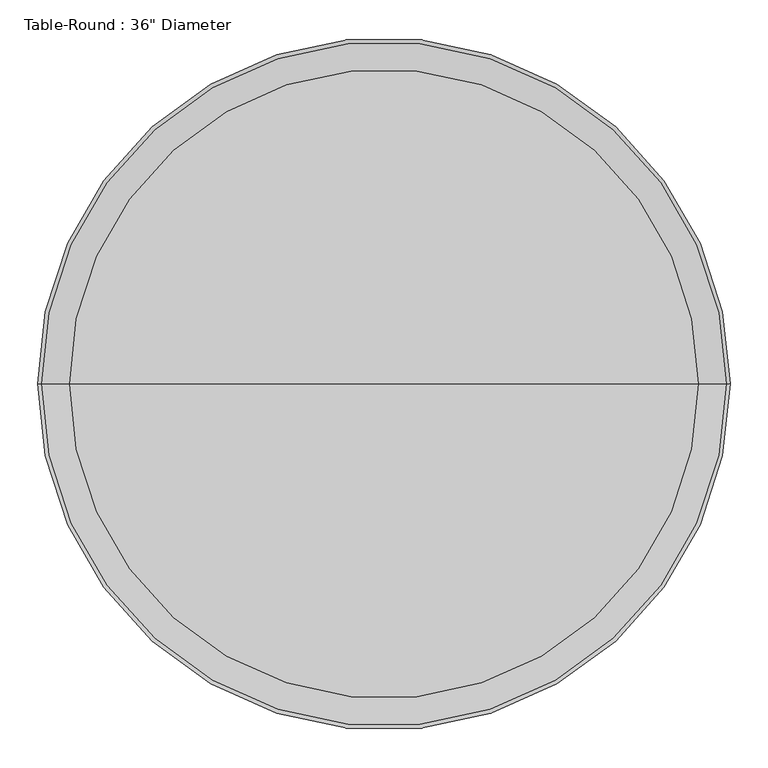
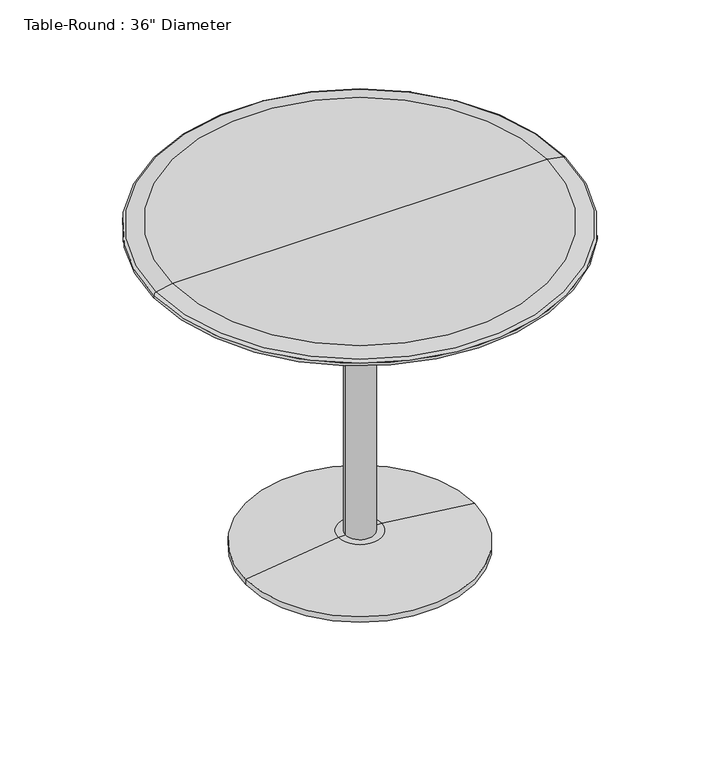
"""IFC4 building model written with IfcOpenShell, lengths in millimetres: furniture geometry."""

from ifc_helpers import new_model, si_unit, point, frame, origin, origin_2d, place, context, project, spatial, polyline, circle_curve, ellipse_curve, trimmed, segment, composite_curve, outline, extrude, source, transform, mapped, element, save
from ifc_brep_helpers import plane_surface, cylinder_surface, revolved_surface, advanced_brep


def furniture_c80d6d9c(model_context):
    return source(origin(), model_context, "Body", "SolidModel", [
        extrude(outline(composite_curve([segment(trimmed(circle_curve(origin_2d(), 31.75), [point((-31.75, 0.0))], [point((31.75, 0.0))], False, "CARTESIAN"), True, "CONTINUOUS"), segment(trimmed(circle_curve(origin_2d(), 31.75), [point((31.75, 0.0))], [point((-31.75, 0.0))], False, "CARTESIAN"), True, "CONTINUOUS")], self_intersect=False)), frame((0.0, 0.0, 38.1), z_axis=(0.0, 0.0, 1.0), x_axis=(1.0, 0.0, 0.0)), (0.0, 0.0, 1.0), 704.85),
        advanced_brep(
        [(0.0, 0.0, 742.95), (-457.2, 0.0, 742.95), (457.2, 0.0, 742.95), (415.3011364, 0.0, 762.0), (-415.3011364, 0.0, 762.0), (0.0, 0.0, 762.0), (451.9526659, 0.0, 755.5373465), (-451.9526659, 0.0, 755.5373465), (457.2, 0.0, 749.2838172), (-457.2, 0.0, 749.2838172)],
        [
            (0, 1),
            (1, 2, circle_curve(frame((0.0, 0.0, 742.95), z_axis=(0.0, 0.0, -1.0), x_axis=(-1.0, 0.0, 0.0)), 457.2)),
            (2, 0),
            (2, 1, circle_curve(frame((0.0, 0.0, 742.95), z_axis=(0.0, 0.0, -1.0), x_axis=(-1.0, 0.0, 0.0)), 457.2)),
            (3, 4, circle_curve(frame((0.0, 0.0, 762.0), z_axis=(0.0, 0.0, 1.0), x_axis=(-1.0, 0.0, 0.0)), 415.3011364)),
            (4, 5),
            (5, 3),
            (4, 3, circle_curve(frame((0.0, 0.0, 762.0), z_axis=(0.0, 0.0, 1.0), x_axis=(-1.0, 0.0, 0.0)), 415.3011364)),
            (6, 7, circle_curve(frame((0.0, 0.0, 755.5373465), z_axis=(0.0, 0.0, 1.0), x_axis=(-1.0, 0.0, 0.0)), 451.9526659)),
            (7, 4),
            (3, 6),
            (7, 6, circle_curve(frame((0.0, 0.0, 755.5373465), z_axis=(0.0, 0.0, 1.0), x_axis=(-1.0, 0.0, 0.0)), 451.9526659)),
            (8, 9, circle_curve(frame((0.0, 0.0, 749.2838172), z_axis=(0.0, 0.0, 1.0), x_axis=(-1.0, 0.0, 0.0)), 457.2)),
            (9, 7, circle_curve(frame((-450.85, 0.0, 749.2838172), z_axis=(0.0, 1.0, 0.0), x_axis=(1.0, 0.0, 0.0)), 6.35)),
            (6, 8, circle_curve(frame((450.85, 0.0, 749.2838172), z_axis=(0.0, 1.0, 0.0), x_axis=(-1.0, 0.0, 0.0)), 6.35)),
            (9, 8, circle_curve(frame((0.0, 0.0, 749.2838172), z_axis=(0.0, 0.0, 1.0), x_axis=(-1.0, 0.0, 0.0)), 457.2)),
            (1, 9),
            (8, 2),
        ],
        [
            plane_surface(frame((0.0, 0.0, 742.95), z_axis=(0.0, 0.0, -1.0), x_axis=(-1.0, 0.0, 0.0))),
            plane_surface(frame((0.0, 0.0, 762.0), z_axis=(0.0, 0.0, 1.0), x_axis=(-1.0, 0.0, 0.0))),
            revolved_surface(polyline([(-415.3011364, 0.0, 762.0), (-451.9526659, 0.0, 755.5373465)]), (0.0, 0.0, 838.2), (0.0, 0.0, -1.0)),
            revolved_surface(trimmed(ellipse_curve(frame((-450.85, 0.0, 749.2838172), z_axis=(0.0, -1.0, 0.0), x_axis=(1.0, 0.0, 0.0)), 6.35, 6.35), [point((-451.9526659, 0.0, 755.5373465))], [point((-457.2, 0.0, 749.2838172))], True, "CARTESIAN"), (0.0, 0.0, 838.2), (0.0, 0.0, -1.0)),
            cylinder_surface(frame((0.0, 0.0, 838.2), z_axis=(0.0, 0.0, -1.0), x_axis=(-1.0, 0.0, 0.0)), 457.2),
        ],
        [
            (0, [[1, 2, 3]]),
            (0, [[-3, 4, -1]]),
            (1, [[5, 6, 7]]),
            (1, [[8, -7, -6]]),
            (2, [[9, 10, -5, 11]]),
            (2, [[12, -11, -8, -10]]),
            (3, [[13, 14, -9, 15]]),
            (3, [[16, -15, -12, -14]]),
            (4, [[-2, 17, -13, 18]]),
            (4, [[-4, -18, -16, -17]]),
        ],
    ),
        advanced_brep(
        [(0.0, 0.0, 0.0), (-254.0, 0.0, 0.0), (254.0, 0.0, 0.0), (47.625, 0.0, 38.1), (-47.625, 0.0, 38.1), (0.0, 0.0, 38.1), (254.0, 0.0, 12.7), (-254.0, 0.0, 12.7)],
        [
            (0, 1),
            (1, 2, circle_curve(frame((0.0, 0.0, 0.0), z_axis=(0.0, 0.0, -1.0), x_axis=(-1.0, 0.0, 0.0)), 254.0)),
            (2, 0),
            (2, 1, circle_curve(frame((0.0, 0.0, 0.0), z_axis=(0.0, 0.0, -1.0), x_axis=(-1.0, 0.0, 0.0)), 254.0)),
            (3, 4, circle_curve(frame((0.0, 0.0, 38.1), z_axis=(0.0, 0.0, 1.0), x_axis=(-1.0, 0.0, 0.0)), 47.625)),
            (4, 5),
            (5, 3),
            (4, 3, circle_curve(frame((0.0, 0.0, 38.1), z_axis=(0.0, 0.0, 1.0), x_axis=(-1.0, 0.0, 0.0)), 47.625)),
            (6, 7, circle_curve(frame((0.0, 0.0, 12.7), z_axis=(0.0, 0.0, 1.0), x_axis=(-1.0, 0.0, 0.0)), 254.0)),
            (7, 4),
            (3, 6),
            (7, 6, circle_curve(frame((0.0, 0.0, 12.7), z_axis=(0.0, 0.0, 1.0), x_axis=(-1.0, 0.0, 0.0)), 254.0)),
            (1, 7),
            (6, 2),
        ],
        [
            plane_surface(frame((0.0, 0.0, 0.0), z_axis=(0.0, 0.0, -1.0), x_axis=(-1.0, 0.0, 0.0))),
            plane_surface(frame((0.0, 0.0, 38.1), z_axis=(0.0, 0.0, 1.0), x_axis=(-1.0, 0.0, 0.0))),
            revolved_surface(polyline([(-47.625, 0.0, 38.1), (-254.0, 0.0, 12.7)]), (0.0, 0.0, 215.9), (0.0, 0.0, -1.0)),
            cylinder_surface(frame((0.0, 0.0, 215.9), z_axis=(0.0, 0.0, -1.0), x_axis=(-1.0, 0.0, 0.0)), 254.0),
        ],
        [
            (0, [[1, 2, 3]]),
            (0, [[-3, 4, -1]]),
            (1, [[5, 6, 7]]),
            (1, [[8, -7, -6]]),
            (2, [[9, 10, -5, 11]]),
            (2, [[12, -11, -8, -10]]),
            (3, [[-2, 13, -9, 14]]),
            (3, [[-4, -14, -12, -13]]),
        ],
    ),
    ])


if __name__ == "__main__":
    model = new_model("IFC4")
    model_context = context("Model", 3, world=origin())
    ifc_project = project(units=[si_unit("LENGTHUNIT", "METRE", prefix="MILLI")], contexts=[model_context])
    site = spatial("IfcSite", under=ifc_project)
    building = spatial("IfcBuilding", under=site)
    placement = place(None, origin())
    furniture_shape = furniture_c80d6d9c(model_context)
    element("IfcFurniture", 1, ObjectType="Table-Round : 36\" Diameter", at=placement, inside=building, context=model_context, shape_type="MappedRepresentation", body=[
        mapped(furniture_shape, transform((0.0, 0.0, 0.0), x_axis=(1.0, 0.0, 0.0), y_axis=(0.0, 1.0, 0.0), z_axis=(0.0, 0.0, 1.0))),
    ])
    save(model, "model.ifc")

# Revit data of these elements
# Type "Table-Round : 36\" Diameter"
#   Assembly Code = "E2020200"
#   Base Radius = 0' - 10"
#   Height = 2' - 6"
#   Radius = 1' - 6"
#   Base Material = Steel, Chrome Plated
#   Top Material = Birch
#   Default Elevation = 0
# Element 1 (IfcFurniture, "Table-Round : 36\" Diameter")
#   Materials on its faces: "Steel, Chrome Plated", "Birch"
# Materials
#   "Steel, Chrome Plated": class "Metal", colour RGB 17 17 17, transparency 0, Description = "Chromiuim plated steel", Cost = 0
#   "Birch": class "Wood", colour RGB 224 178 126, transparency 0, Description = "Betula Alleghaniensis", Cost = 0
